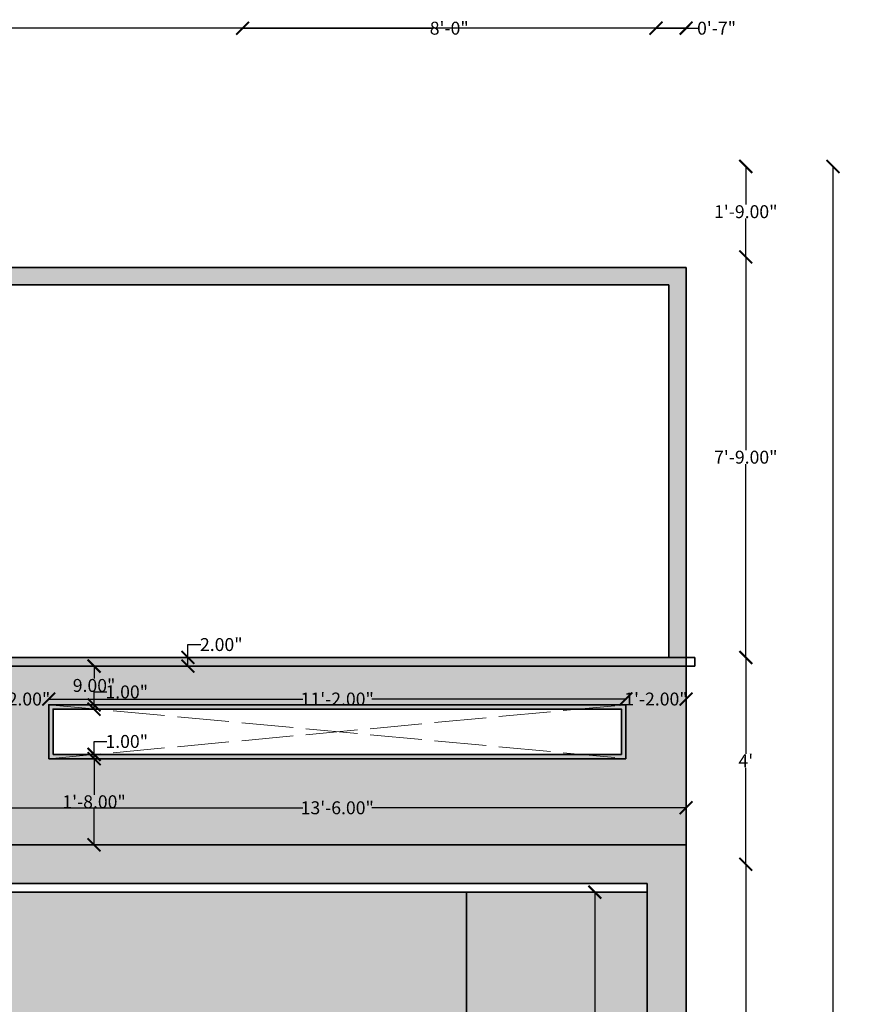
# Model space of a CAD drawing. Units: inches. Extents: x -654 to 390, y -40 to 648.
# Tile 13 of 13: x 192 to 386, y 417 to 645. Entities that reach past the tile are written whole.
import ezdxf

# ---------------------------------------------------------------- set-up
doc = ezdxf.new("R2010")
doc.units = ezdxf.units.IN
doc.header["$PDMODE"] = 3
doc.linetypes.add('ACAD_ISO02W100', pattern=[15, 12, -3])
for name, color, linetype, lineweight in [('A-ANNO-DIMS', 2, 'Continuous', 18), ('A-ELEV', 7, 'Continuous', 35), ('A-ELEV-FILL', 252, 'Continuous', 13), ('A-ELEV-HIDN', 8, 'ACAD_ISO02W100', 18)]:
    doc.layers.add(name, color=color, linetype=linetype, lineweight=lineweight)
doc.styles.get("Standard").update_dxf_attribs({"font": 'arial.ttf'})
doc.dimstyles.get("Standard").update_dxf_attribs({"dimtxt": 3, "dimasz": 3, "dimexe": 0.18, "dimexo": 0.0625, "dimgap": 0.09, "dimtad": 0, "dimtih": 1, "dimtoh": 1, "dimzin": 0, "dimdsep": 46, "dimlunit": 3, "dimtxsty": 'Standard', "dimblk": 'ARCHTICK', "dimcen": 0.09, "dimse1": 1, "dimse2": 1, "dimadec": 0, "dimazin": 0, "dimtfac": 1, "dimtofl": 0, "dimtmove": 0, "dimatfit": 3, "dimfxl": 1, "dimtolj": 1, "dimtzin": 0, "dimarcsym": 0})

# ---------------------------------------------------------------- blocks, each defined once
blk = doc.blocks.new('_ArchTick')
at = {"color": 0, "linetype": 'ByBlock', "const_width": 0.15}
blk.add_lwpolyline([(-0.5, -0.5), (0.5, 0.5)], dxfattribs=at)
blk = doc.blocks.new('*D6')
at = {"layer": 'A-ANNO-DIMS', "color": 0, "lineweight": -2, "transparency": 16777216}
for p, q in [((360.51, 449.13), (360.51, 381.76)), ((360.51, 311.13), (360.51, 378.51))]:
    blk.add_line(p, q, dxfattribs=at)
at = {"layer": 'Defpoints', "color": 0, "transparency": 16777216}
for p in [(337.55, 449.13), (360.51, 449.13), (303.82, 311.13)]:
    blk.add_point(p, dxfattribs=at)
at = {"layer": 'A-ANNO-DIMS', "color": 0, "lineweight": -2, "transparency": 16777216, "xscale": 3, "yscale": 3, "zscale": 3}
for p, rotation in [((360.51, 449.13), 90), ((360.51, 311.13), 270)]:
    blk.add_blockref('_ArchTick', p, dxfattribs=dict(at, rotation=rotation))
at = {"layer": 'A-ANNO-DIMS', "color": 0, "transparency": 16777216, "insert": (360.51, 380.13), "char_height": 3, "attachment_point": 5}
blk.add_mtext('\\A1;11\'-6.00"', dxfattribs=at)
blk = doc.blocks.new('*D7')
at = {"layer": 'A-ANNO-DIMS', "color": 0, "lineweight": -2, "transparency": 16777216}
for p, q in [((360.51, 497.13), (360.51, 474.72)), ((360.51, 449.13), (360.51, 471.54))]:
    blk.add_line(p, q, dxfattribs=at)
at = {"layer": 'Defpoints', "color": 0, "transparency": 16777216}
for p in [(346.65, 497.13), (360.51, 497.13), (337.55, 449.13)]:
    blk.add_point(p, dxfattribs=at)
at = {"layer": 'A-ANNO-DIMS', "color": 0, "lineweight": -2, "transparency": 16777216, "xscale": 3, "yscale": 3, "zscale": 3}
for p, rotation in [((360.51, 497.13), 90), ((360.51, 449.13), 270)]:
    blk.add_blockref('_ArchTick', p, dxfattribs=dict(at, rotation=rotation))
at = {"layer": 'A-ANNO-DIMS', "color": 0, "transparency": 16777216, "insert": (360.51, 473.13), "char_height": 3, "attachment_point": 5}
blk.add_mtext("\\A1;4'", dxfattribs=at)
blk = doc.blocks.new('*D8')
at = {"layer": 'A-ANNO-DIMS', "color": 0, "lineweight": -2, "transparency": 16777216}
for p, q in [((360.51, 590.13), (360.51, 545.26)), ((360.51, 497.13), (360.51, 542.01))]:
    blk.add_line(p, q, dxfattribs=at)
at = {"layer": 'Defpoints', "color": 0, "transparency": 16777216}
for p in [(161.04, 590.13), (360.51, 590.13), (346.65, 497.13)]:
    blk.add_point(p, dxfattribs=at)
at = {"layer": 'A-ANNO-DIMS', "color": 0, "lineweight": -2, "transparency": 16777216, "xscale": 3, "yscale": 3, "zscale": 3}
for p, rotation in [((360.51, 590.13), 90), ((360.51, 497.13), 270)]:
    blk.add_blockref('_ArchTick', p, dxfattribs=dict(at, rotation=rotation))
at = {"layer": 'A-ANNO-DIMS', "color": 0, "transparency": 16777216, "insert": (360.51, 543.63), "char_height": 3, "attachment_point": 5}
blk.add_mtext('\\A1;7\'-9.00"', dxfattribs=at)
blk = doc.blocks.new('*D9')
at = {"layer": 'A-ANNO-DIMS', "color": 0, "lineweight": -2, "transparency": 16777216}
for p, q in [((360.51, 611.13), (360.51, 602.26)), ((360.51, 590.13), (360.51, 599.01))]:
    blk.add_line(p, q, dxfattribs=at)
at = {"layer": 'Defpoints', "color": 0, "transparency": 16777216}
for p in [(126.65, 611.13), (360.51, 611.13), (161.04, 590.13)]:
    blk.add_point(p, dxfattribs=at)
at = {"layer": 'A-ANNO-DIMS', "color": 0, "lineweight": -2, "transparency": 16777216, "xscale": 3, "yscale": 3, "zscale": 3}
for p, rotation in [((360.51, 611.13), 90), ((360.51, 590.13), 270)]:
    blk.add_blockref('_ArchTick', p, dxfattribs=dict(at, rotation=rotation))
at = {"layer": 'A-ANNO-DIMS', "color": 0, "transparency": 16777216, "insert": (360.51, 600.63), "char_height": 3, "attachment_point": 5}
blk.add_mtext('\\A1;1\'-9.00"', dxfattribs=at)
blk = doc.blocks.new('*D32')
at = {"layer": 'A-ANNO-DIMS', "color": 0, "lineweight": -2, "transparency": 16777216}
for p, q in [((184.65, 462.23), (257.63, 462.23)), ((346.65, 462.23), (273.66, 462.23))]:
    blk.add_line(p, q, dxfattribs=at)
at = {"layer": 'Defpoints', "color": 0, "transparency": 16777216}
for p in [(184.65, 462.23), (346.65, 462.23), (346.65, 462.23)]:
    blk.add_point(p, dxfattribs=at)
at = {"layer": 'A-ANNO-DIMS', "color": 0, "lineweight": -2, "transparency": 16777216, "xscale": 3, "yscale": 3, "zscale": 3, "rotation": 180}
blk.add_blockref('_ArchTick', (184.65, 462.23), dxfattribs=at)
at = {"layer": 'A-ANNO-DIMS', "color": 0, "lineweight": -2, "transparency": 16777216, "xscale": 3, "yscale": 3, "zscale": 3}
blk.add_blockref('_ArchTick', (346.65, 462.23), dxfattribs=at)
at = {"layer": 'A-ANNO-DIMS', "color": 0, "transparency": 16777216, "insert": (265.65, 462.23), "char_height": 3, "attachment_point": 5}
blk.add_mtext('\\A1;13\'-6.00"', dxfattribs=at)
blk = doc.blocks.new('*D33')
at = {"layer": 'A-ANNO-DIMS', "color": 0, "lineweight": -2, "transparency": 16777216}
for p, q in [((209.18, 473.63), (209.18, 465.26)), ((209.18, 453.63), (209.18, 462.01))]:
    blk.add_line(p, q, dxfattribs=at)
at = {"layer": 'Defpoints', "color": 0, "transparency": 16777216}
for p in [(198.65, 473.63), (198.65, 453.63), (209.18, 453.63)]:
    blk.add_point(p, dxfattribs=at)
at = {"layer": 'A-ANNO-DIMS', "color": 0, "lineweight": -2, "transparency": 16777216, "xscale": 3, "yscale": 3, "zscale": 3}
for p, rotation in [((209.18, 473.63), 90), ((209.18, 453.63), 270)]:
    blk.add_blockref('_ArchTick', p, dxfattribs=dict(at, rotation=rotation))
at = {"layer": 'A-ANNO-DIMS', "color": 0, "transparency": 16777216, "insert": (209.18, 463.63), "char_height": 3, "attachment_point": 5}
blk.add_mtext('\\A1;1\'-8.00"', dxfattribs=at)
blk = doc.blocks.new('*D34')
at = {"layer": 'A-ANNO-DIMS', "color": 0, "lineweight": -2, "transparency": 16777216}
for p, q in [((209.18, 474.63), (209.18, 477.63)), ((209.18, 477.63), (212.18, 477.63)), ((209.18, 473.63), (209.18, 474.63))]:
    blk.add_line(p, q, dxfattribs=at)
at = {"layer": 'Defpoints', "color": 0, "transparency": 16777216}
for p in [(209.18, 474.63), (209.18, 474.63), (209.18, 473.63)]:
    blk.add_point(p, dxfattribs=at)
at = {"layer": 'A-ANNO-DIMS', "color": 0, "lineweight": -2, "transparency": 16777216, "xscale": 3, "yscale": 3, "zscale": 3}
for p, rotation in [((209.18, 474.63), 90), ((209.18, 473.63), 270)]:
    blk.add_blockref('_ArchTick', p, dxfattribs=dict(at, rotation=rotation))
at = {"layer": 'A-ANNO-DIMS', "color": 0, "transparency": 16777216, "insert": (216.77, 477.63), "char_height": 3, "attachment_point": 5}
blk.add_mtext('\\A1;1.00"', dxfattribs=at)
blk = doc.blocks.new('*D35')
at = {"layer": 'A-ANNO-DIMS', "color": 0, "lineweight": -2, "transparency": 16777216}
for p, q in [((209.18, 486.13), (209.18, 489.13)), ((209.18, 489.13), (212.18, 489.13)), ((209.18, 485.13), (209.18, 486.13))]:
    blk.add_line(p, q, dxfattribs=at)
at = {"layer": 'Defpoints', "color": 0, "transparency": 16777216}
for p in [(209.18, 486.13), (209.37, 486.13), (209.37, 485.13)]:
    blk.add_point(p, dxfattribs=at)
at = {"layer": 'A-ANNO-DIMS', "color": 0, "lineweight": -2, "transparency": 16777216, "xscale": 3, "yscale": 3, "zscale": 3}
for p, rotation in [((209.18, 486.13), 90), ((209.18, 485.13), 270)]:
    blk.add_blockref('_ArchTick', p, dxfattribs=dict(at, rotation=rotation))
at = {"layer": 'A-ANNO-DIMS', "color": 0, "transparency": 16777216, "insert": (216.77, 489.13), "char_height": 3, "attachment_point": 5}
blk.add_mtext('\\A1;1.00"', dxfattribs=at)
blk = doc.blocks.new('*D36')
at = {"layer": 'A-ANNO-DIMS', "color": 0, "lineweight": -2, "transparency": 16777216}
for p, q in [((209.18, 495.13), (209.18, 492.26)), ((209.18, 486.13), (209.18, 489.01))]:
    blk.add_line(p, q, dxfattribs=at)
at = {"layer": 'Defpoints', "color": 0, "transparency": 16777216}
for p in [(198.65, 495.13), (209.18, 495.13), (198.65, 486.13)]:
    blk.add_point(p, dxfattribs=at)
at = {"layer": 'A-ANNO-DIMS', "color": 0, "lineweight": -2, "transparency": 16777216, "xscale": 3, "yscale": 3, "zscale": 3}
for p, rotation in [((209.18, 495.13), 90), ((209.18, 486.13), 270)]:
    blk.add_blockref('_ArchTick', p, dxfattribs=dict(at, rotation=rotation))
at = {"layer": 'A-ANNO-DIMS', "color": 0, "transparency": 16777216, "insert": (209.18, 490.63), "char_height": 3, "attachment_point": 5}
blk.add_mtext('\\A1;9.00"', dxfattribs=at)
blk = doc.blocks.new('*D37')
at = {"layer": 'A-ANNO-DIMS', "color": 0, "lineweight": -2, "transparency": 16777216}
for p, q in [((184.65, 487.48), (184.8, 487.48)), ((198.65, 487.48), (198.5, 487.48))]:
    blk.add_line(p, q, dxfattribs=at)
at = {"layer": 'Defpoints', "color": 0, "transparency": 16777216}
for p in [(184.65, 487.48), (184.65, 486.13), (198.65, 486.13)]:
    blk.add_point(p, dxfattribs=at)
at = {"layer": 'A-ANNO-DIMS', "color": 0, "lineweight": -2, "transparency": 16777216, "xscale": 3, "yscale": 3, "zscale": 3, "rotation": 180}
blk.add_blockref('_ArchTick', (184.65, 487.48), dxfattribs=at)
at = {"layer": 'A-ANNO-DIMS', "color": 0, "lineweight": -2, "transparency": 16777216, "xscale": 3, "yscale": 3, "zscale": 3}
blk.add_blockref('_ArchTick', (198.65, 487.48), dxfattribs=at)
at = {"layer": 'A-ANNO-DIMS', "color": 0, "transparency": 16777216, "insert": (191.65, 487.48), "char_height": 3, "attachment_point": 5}
blk.add_mtext('\\A1;1\'-2.00"', dxfattribs=at)
blk = doc.blocks.new('*D38')
at = {"layer": 'A-ANNO-DIMS', "color": 0, "lineweight": -2, "transparency": 16777216}
for p, q in [((198.65, 487.48), (257.63, 487.48)), ((332.65, 487.48), (273.66, 487.48))]:
    blk.add_line(p, q, dxfattribs=at)
at = {"layer": 'Defpoints', "color": 0, "transparency": 16777216}
for p in [(332.65, 487.48), (198.65, 486.13), (332.65, 486.13)]:
    blk.add_point(p, dxfattribs=at)
at = {"layer": 'A-ANNO-DIMS', "color": 0, "lineweight": -2, "transparency": 16777216, "xscale": 3, "yscale": 3, "zscale": 3, "rotation": 180}
blk.add_blockref('_ArchTick', (198.65, 487.48), dxfattribs=at)
at = {"layer": 'A-ANNO-DIMS', "color": 0, "lineweight": -2, "transparency": 16777216, "xscale": 3, "yscale": 3, "zscale": 3}
blk.add_blockref('_ArchTick', (332.65, 487.48), dxfattribs=at)
at = {"layer": 'A-ANNO-DIMS', "color": 0, "transparency": 16777216, "insert": (265.65, 487.48), "char_height": 3, "attachment_point": 5}
blk.add_mtext('\\A1;11\'-2.00"', dxfattribs=at)
blk = doc.blocks.new('*D39')
at = {"layer": 'A-ANNO-DIMS', "color": 0, "lineweight": -2, "transparency": 16777216}
for p, q in [((332.65, 487.48), (332.8, 487.48)), ((346.65, 487.48), (346.5, 487.48))]:
    blk.add_line(p, q, dxfattribs=at)
at = {"layer": 'Defpoints', "color": 0, "transparency": 16777216}
for p in [(346.65, 487.48), (346.65, 487.48), (332.65, 486.13)]:
    blk.add_point(p, dxfattribs=at)
at = {"layer": 'A-ANNO-DIMS', "color": 0, "lineweight": -2, "transparency": 16777216, "xscale": 3, "yscale": 3, "zscale": 3, "rotation": 180}
blk.add_blockref('_ArchTick', (332.65, 487.48), dxfattribs=at)
at = {"layer": 'A-ANNO-DIMS', "color": 0, "lineweight": -2, "transparency": 16777216, "xscale": 3, "yscale": 3, "zscale": 3}
blk.add_blockref('_ArchTick', (346.65, 487.48), dxfattribs=at)
at = {"layer": 'A-ANNO-DIMS', "color": 0, "transparency": 16777216, "insert": (339.65, 487.48), "char_height": 3, "attachment_point": 5}
blk.add_mtext('\\A1;1\'-2.00"', dxfattribs=at)
blk = doc.blocks.new('*D40')
at = {"layer": 'A-ANNO-DIMS', "color": 0, "lineweight": -2, "transparency": 16777216}
for p, q in [((230.97, 497.13), (230.97, 500.13)), ((230.97, 500.13), (233.97, 500.13)), ((230.97, 495.13), (230.97, 497.13))]:
    blk.add_line(p, q, dxfattribs=at)
at = {"layer": 'Defpoints', "color": 0, "transparency": 16777216}
for p in [(182.52, 497.13), (230.97, 497.13), (182.52, 495.13)]:
    blk.add_point(p, dxfattribs=at)
at = {"layer": 'A-ANNO-DIMS', "color": 0, "lineweight": -2, "transparency": 16777216, "xscale": 3, "yscale": 3, "zscale": 3}
for p, rotation in [((230.97, 497.13), 90), ((230.97, 495.13), 270)]:
    blk.add_blockref('_ArchTick', p, dxfattribs=dict(at, rotation=rotation))
at = {"layer": 'A-ANNO-DIMS', "color": 0, "transparency": 16777216, "insert": (238.72, 500.13), "char_height": 3, "attachment_point": 5}
blk.add_mtext('\\A1;2.00"', dxfattribs=at)
blk = doc.blocks.new('*D41')
at = {"layer": 'A-ANNO-DIMS', "color": 0, "lineweight": -2, "transparency": 16777216}
for p, q in [((325.46, 442.63), (325.46, 311.76)), ((325.46, 177.63), (325.46, 308.51))]:
    blk.add_line(p, q, dxfattribs=at)
at = {"layer": 'Defpoints', "color": 0, "transparency": 16777216}
for p in [(295.65, 442.63), (295.65, 177.63), (325.46, 177.63)]:
    blk.add_point(p, dxfattribs=at)
at = {"layer": 'A-ANNO-DIMS', "color": 0, "lineweight": -2, "transparency": 16777216, "xscale": 3, "yscale": 3, "zscale": 3}
for p, rotation in [((325.46, 442.63), 90), ((325.46, 177.63), 270)]:
    blk.add_blockref('_ArchTick', p, dxfattribs=dict(at, rotation=rotation))
at = {"layer": 'A-ANNO-DIMS', "color": 0, "transparency": 16777216, "insert": (325.46, 310.13), "char_height": 3, "attachment_point": 5}
blk.add_mtext('\\A1;22\'-1.00"', dxfattribs=at)
blk = doc.blocks.new('*D75')
at = {"layer": 'A-ANNO-DIMS', "color": 0, "lineweight": -2, "transparency": 16777216}
for p, q in [((-1.35, 643.23), (167.38, 643.23)), ((346.65, 643.23), (177.91, 643.23))]:
    blk.add_line(p, q, dxfattribs=at)
at = {"layer": 'Defpoints', "color": 0, "transparency": 16777216}
for p in [(346.65, 643.23), (-1.35, 611.13), (346.65, 587.63)]:
    blk.add_point(p, dxfattribs=at)
at = {"layer": 'A-ANNO-DIMS', "color": 0, "lineweight": -2, "transparency": 16777216, "xscale": 3, "yscale": 3, "zscale": 3, "rotation": 180}
blk.add_blockref('_ArchTick', (-1.35, 643.23), dxfattribs=at)
at = {"layer": 'A-ANNO-DIMS', "color": 0, "lineweight": -2, "transparency": 16777216, "xscale": 3, "yscale": 3, "zscale": 3}
blk.add_blockref('_ArchTick', (346.65, 643.23), dxfattribs=at)
at = {"layer": 'A-ANNO-DIMS', "color": 0, "transparency": 16777216, "insert": (172.65, 643.23), "char_height": 3, "attachment_point": 5}
blk.add_mtext('\\A1;29\'-0"', dxfattribs=at)
blk = doc.blocks.new('*D76')
at = {"layer": 'A-ANNO-DIMS', "color": 0, "lineweight": -2, "transparency": 16777216}
for p, q in [((380.75, 611.13), (380.75, 306.76)), ((380.75, -0.87), (380.75, 303.51))]:
    blk.add_line(p, q, dxfattribs=at)
at = {"layer": 'Defpoints', "color": 0, "transparency": 16777216}
for p in [(126.65, 611.13), (380.75, 611.13), (346.65, -0.87)]:
    blk.add_point(p, dxfattribs=at)
at = {"layer": 'A-ANNO-DIMS', "color": 0, "lineweight": -2, "transparency": 16777216, "xscale": 3, "yscale": 3, "zscale": 3}
for p, rotation in [((380.75, 611.13), 90), ((380.75, -0.87), 270)]:
    blk.add_blockref('_ArchTick', p, dxfattribs=dict(at, rotation=rotation))
at = {"layer": 'A-ANNO-DIMS', "color": 0, "transparency": 16777216, "insert": (380.75, 305.13), "char_height": 3, "attachment_point": 5}
blk.add_mtext('\\A1;51\'-0"', dxfattribs=at)
blk = doc.blocks.new('*D89')
at = {"layer": 'A-ANNO-DIMS', "color": 0, "lineweight": -2, "transparency": 16777216}
for p, q in [((243.65, 643.23), (287.57, 643.23)), ((339.65, 643.23), (295.73, 643.23))]:
    blk.add_line(p, q, dxfattribs=at)
at = {"layer": 'Defpoints', "color": 0, "transparency": 16777216}
for p in [(339.65, 643.23), (243.65, 17.13), (339.65, 17.13)]:
    blk.add_point(p, dxfattribs=at)
at = {"layer": 'A-ANNO-DIMS', "color": 0, "lineweight": -2, "transparency": 16777216, "xscale": 3, "yscale": 3, "zscale": 3, "rotation": 180}
blk.add_blockref('_ArchTick', (243.65, 643.23), dxfattribs=at)
at = {"layer": 'A-ANNO-DIMS', "color": 0, "lineweight": -2, "transparency": 16777216, "xscale": 3, "yscale": 3, "zscale": 3}
blk.add_blockref('_ArchTick', (339.65, 643.23), dxfattribs=at)
at = {"layer": 'A-ANNO-DIMS', "color": 0, "transparency": 16777216, "insert": (291.65, 643.23), "char_height": 3, "attachment_point": 5}
blk.add_mtext('\\A1;8\'-0"', dxfattribs=at)
blk = doc.blocks.new('*D90')
at = {"layer": 'A-ANNO-DIMS', "color": 0, "lineweight": -2, "transparency": 16777216}
for p, q in [((339.65, 643.23), (346.65, 643.23)), ((346.65, 643.23), (349.65, 643.23))]:
    blk.add_line(p, q, dxfattribs=at)
at = {"layer": 'Defpoints', "color": 0, "transparency": 16777216}
for p in [(346.65, 643.23), (339.65, 17.13), (346.65, 17.13)]:
    blk.add_point(p, dxfattribs=at)
at = {"layer": 'A-ANNO-DIMS', "color": 0, "lineweight": -2, "transparency": 16777216, "xscale": 3, "yscale": 3, "zscale": 3, "rotation": 180}
blk.add_blockref('_ArchTick', (339.65, 643.23), dxfattribs=at)
at = {"layer": 'A-ANNO-DIMS', "color": 0, "lineweight": -2, "transparency": 16777216, "xscale": 3, "yscale": 3, "zscale": 3}
blk.add_blockref('_ArchTick', (346.65, 643.23), dxfattribs=at)
at = {"layer": 'A-ANNO-DIMS', "color": 0, "transparency": 16777216, "insert": (353.72, 643.23), "char_height": 3, "attachment_point": 5}
blk.add_mtext('\\A1;0\'-7"', dxfattribs=at)

msp = doc.modelspace()

# ---------------------------------------------------------------- hatches: boundary and pattern name
at = {"layer": 'A-ELEV-FILL'}
h = msp.add_hatch(color=256, dxfattribs=at)
h.dxf.hatch_style = 1
h.paths.add_polyline_path([(126.646, 611.134), (124.646, 611.134), (-1.354, 611.134), (-3.354, 611.134), (-3.354, 609.134), (-1.354, 609.134), (124.646, 609.134), (126.646, 609.134)])
h.paths.add_polyline_path([(8.646, 497.134), (-2.354, 497.134), (-2.354, 495.134), (8.646, 495.134)])
h.paths.add_polyline_path([(346.646, 497.134), (182.515, 497.134), (182.515, 495.134), (346.646, 495.134)])
h.paths.add_polyline_path([(198.646, 486.134), (198.646, 473.634), (209.366, 474.634), (199.646, 474.634), (199.646, 485.134), (209.366, 485.134)])
h.paths.add_polyline_path([(332.646, 486.134), (198.646, 486.134), (209.366, 485.134), (321.926, 485.134)])
h.paths.add_polyline_path([(321.926, 474.634), (209.366, 474.634), (198.646, 473.634), (332.646, 473.634)])
h.paths.add_polyline_path([(332.646, 486.134), (321.926, 485.134), (331.646, 485.134), (331.646, 474.634), (321.926, 474.634), (332.646, 473.634)])
h = msp.add_hatch(color=256, dxfattribs=at)
h.dxf.hatch_style = 1
h.paths.add_polyline_path([(161.035, 590.134), (-1.354, 590.134), (-1.354, 581.134), (161.035, 581.134)])
h.paths.add_polyline_path([(346.646, 453.634), (-1.354, 453.634), (-1.354, 444.634), (337.646, 444.634), (337.646, 177.634), (178.742, 177.634), (178.742, 173.134), (176.742, 173.134), (176.742, 177.634), (166.742, 177.634), (166.742, 173.134), (164.742, 173.134), (164.742, 177.634), (154.742, 177.634), (154.742, 173.134), (152.742, 173.134), (152.742, 177.634), (142.742, 177.634), (142.742, 173.134), (140.742, 173.134), (140.742, 177.634), (130.742, 177.634), (130.742, 173.134), (128.742, 173.134), (128.742, 177.634), (115.646, 177.634), (115.646, 168.634), (346.646, 168.634), (346.646, 173.134)])
h.paths.add_polyline_path([(7.646, 87.642), (-1.354, 87.642), (-1.354, 17.134), (7.646, 17.134)])
h.paths.add_polyline_path([(16.396, 116.134), (60.646, 116.134), (60.646, 83.134), (62.646, 83.134), (113.646, 83.134), (115.646, 83.134), (115.646, 125.134), (7.646, 125.134), (7.646, 89.642), (8.146, 89.642), (8.146, 87.642), (7.646, 87.642), (7.646, 83.134), (9.646, 83.134), (16.396, 83.134)])
h = msp.add_hatch(color=256, dxfattribs=at)
h.dxf.hatch_style = 1
h.paths.add_polyline_path([(346.646, 587.634), (161.035, 587.634), (161.035, 583.634), (342.646, 583.634), (342.646, 497.134), (346.646, 497.134), (346.646, 583.634)])
h.paths.add_polyline_path([(295.646, 315.634), (98.293, 315.634), (98.293, 311.134), (295.646, 311.134)])
h.paths.add_polyline_path([(128.742, 311.134), (98.293, 311.134), (98.293, 306.634), (128.742, 306.634)])
h.paths.add_polyline_path([(140.742, 311.134), (130.742, 311.134), (130.742, 306.634), (140.742, 306.634)])
h.paths.add_polyline_path([(152.742, 311.134), (142.742, 311.134), (142.742, 306.634), (152.742, 306.634)])
h.paths.add_polyline_path([(164.742, 311.134), (154.742, 311.134), (154.742, 306.634), (164.742, 306.634)])
h.paths.add_polyline_path([(176.742, 311.134), (166.742, 311.134), (166.742, 306.634), (176.742, 306.634)])
h.paths.add_polyline_path([(295.646, 311.134), (178.742, 311.134), (178.742, 306.634), (295.646, 306.634)])
h.paths.add_polyline_path([(303.818, 315.634), (295.646, 315.634), (295.646, 311.134), (303.818, 311.134)])
h.paths.add_polyline_path([(303.818, 311.134), (295.646, 311.134), (295.646, 306.634), (303.818, 306.634)])
h = msp.add_hatch(color=256, dxfattribs=at)
h.dxf.hatch_style = 1
h.paths.add_polyline_path([(41.55, 80.08), (28.05, 80.08), (28.05, 20.08), (41.55, 20.08)])
h.paths.add_polyline_path([(93.843, 80.08), (80.343, 80.08), (80.343, 20.08), (93.843, 20.08)])
h.paths.add_polyline_path([(337.646, 442.634), (295.646, 442.634), (295.646, 316.634), (304.646, 316.634), (304.646, 315.634), (303.818, 315.634), (303.818, 306.634), (304.646, 306.634), (304.646, 305.634), (295.646, 305.634), (295.646, 177.634), (337.646, 177.634)])
h.paths.add_polyline_path([(346.646, 495.134), (184.646, 495.134), (184.646, 453.634), (346.646, 453.634)])
h.paths.add_polyline_path([(198.646, 473.634), (198.646, 486.134), (332.646, 486.134), (332.646, 473.634)], flags=16)
h.paths.add_polyline_path([(199.646, 474.634), (199.646, 485.134), (331.646, 485.134), (331.646, 474.634)], flags=0)
h = msp.add_hatch(color=256, dxfattribs=at)
h.dxf.hatch_style = 1
h.paths.add_polyline_path([(239.871, 410.786), (291.141, 410.786), (291.141, 355.634), (295.646, 355.634), (295.646, 442.634), (145.646, 442.634), (145.646, 410.786), (179.877, 410.786), (179.877, 355.634), (239.871, 355.634)])

# ---------------------------------------------------------------- linework, layer by layer
at = {"layer": 'A-ELEV'}
for p, q in [((161.035, 587.634), (346.646, 587.634)), ((346.646, -0.866), (346.646, 587.634)), ((161.035, 583.634), (342.646, 583.634)), ((342.646, 583.634), (342.646, 497.134)), ((346.646, 583.634), (346.646, 497.134)), ((182.515, 497.134), (348.646, 497.134)), ((348.646, 495.134), (348.646, 497.134)), ((182.515, 495.134), (348.646, 495.134)), ((-1.354, 453.634), (346.646, 453.634)), ((-1.354, 444.634), (337.646, 444.634)), ((337.646, 444.634), (337.646, 177.634)), ((-1.354, 442.634), (337.646, 442.634)), ((295.646, 442.634), (295.646, 177.634))]:
    msp.add_line(p, q, dxfattribs=at)
for points in [[(198.646, 473.634), (198.646, 486.134), (332.646, 486.134), (332.646, 473.634)], [(199.646, 474.634), (199.646, 485.134), (331.646, 485.134), (331.646, 474.634)]]:
    msp.add_lwpolyline(points, close=True, dxfattribs=at)
at = {"layer": 'A-ELEV-HIDN'}
for p, q in [((198.646, 486.134), (332.646, 473.634)), ((198.646, 473.634), (332.646, 486.134))]:
    msp.add_line(p, q, dxfattribs=at)

# ---------------------------------------------------------------- dimensions: what is measured, and where the dimension line sits
at = {"layer": 'A-ANNO-DIMS'}
for base, p1, p2, override, picture, middle in [((346.646, 643.234), (-1.354, 611.134), (346.646, 587.634), {"dimdec": 1, "dimlfac": 1, "dimrnd": 0, "dimzin": 1, "dimdsep": 46, "dimlunit": 4, "dimfrac": 2}, '*D75', (172.646, 643.234)), ((339.646, 643.234), (243.646, 17.134), (339.646, 17.134), {"dimdec": 1, "dimlfac": 1, "dimrnd": 0, "dimzin": 1, "dimdsep": 46, "dimlunit": 4, "dimfrac": 2}, '*D89', (291.646, 643.234)), ((346.646, 643.234), (339.646, 17.134), (346.646, 17.134), {"dimdec": 1, "dimlfac": 1, "dimrnd": 0, "dimzin": 1, "dimdsep": 46, "dimlunit": 4, "dimfrac": 2}, '*D90', (353.724, 643.234)), ((184.646, 487.476), (198.646, 486.134), (184.646, 486.134), {"dimclrd": 0, "dimclre": 0, "dimclrt": 0}, '*D37', (191.646, 487.476)), ((332.646, 487.476), (198.646, 486.134), (332.646, 486.134), {"dimclrd": 0, "dimclre": 0, "dimclrt": 0}, '*D38', (265.646, 487.476)), ((346.646, 487.476), (332.646, 486.134), (346.646, 487.476), {"dimclrd": 0, "dimclre": 0, "dimclrt": 0, "dimtmove": 1}, '*D39', (339.646, 487.476)), ((346.646, 462.232), (184.646, 462.232), (346.646, 462.232), {"dimclrd": 0, "dimclre": 0, "dimclrt": 0, "dimtmove": 1}, '*D32', (265.646, 462.232))]:
    dim = msp.add_linear_dim(base=base, p1=p1, p2=p2, dimstyle='Standard', override=override, dxfattribs=at)
    dim.commit()
    dim.dimension.update_dxf_attribs({"geometry": picture, "text_midpoint": middle})
for base, p1, p2, override, picture, middle in [((360.508, 611.134), (161.035, 590.134), (126.646, 611.134), {"dimclrd": 0, "dimclre": 0, "dimclrt": 0, "dimtmove": 1}, '*D9', (360.508, 600.634)), ((380.746, 611.134), (346.646, -0.866), (126.646, 611.134), {"dimdec": 1, "dimlfac": 1, "dimrnd": 0, "dimzin": 1, "dimdsep": 46, "dimlunit": 4, "dimfrac": 2}, '*D76', (380.746, 305.134)), ((360.508, 590.134), (346.646, 497.134), (161.035, 590.134), {"dimclrd": 0, "dimclre": 0, "dimclrt": 0, "dimtmove": 1}, '*D8', (360.508, 543.634)), ((230.972, 497.134), (182.515, 495.134), (182.515, 497.134), {"dimclrd": 0, "dimclre": 0, "dimclrt": 0}, '*D40', (238.724, 500.134)), ((360.508, 497.134), (337.554, 449.134), (346.646, 497.134), {"dimclrd": 0, "dimclre": 0, "dimclrt": 0, "dimtmove": 1}, '*D7', (360.508, 473.134)), ((209.184, 495.134), (198.646, 486.134), (198.646, 495.134), {"dimclrd": 0, "dimclre": 0, "dimclrt": 0}, '*D36', (209.184, 490.634)), ((209.184, 486.134), (209.366, 485.134), (209.366, 486.134), {"dimclrd": 0, "dimclre": 0, "dimclrt": 0}, '*D35', (216.77, 489.134)), ((209.184, 474.634), (209.184, 473.634), (209.184, 474.634), {"dimclrd": 0, "dimclre": 0, "dimclrt": 0}, '*D34', (216.77, 477.634)), ((209.184, 453.634), (198.646, 473.634), (198.646, 453.634), {"dimclrd": 0, "dimclre": 0, "dimclrt": 0}, '*D33', (209.184, 463.634)), ((360.508, 449.134), (303.818, 311.134), (337.554, 449.134), {"dimclrd": 0, "dimclre": 0, "dimclrt": 0, "dimtmove": 1}, '*D6', (360.508, 380.134)), ((325.461, 177.634), (295.646, 442.634), (295.646, 177.634), {"dimclrd": 0, "dimclre": 0, "dimclrt": 0}, '*D41', (325.461, 310.134))]:
    dim = msp.add_linear_dim(base=base, p1=p1, p2=p2, angle=90, dimstyle='Standard', override=override, dxfattribs=at)
    dim.commit()
    dim.dimension.update_dxf_attribs({"geometry": picture, "text_midpoint": middle})

doc.saveas('drawing.dxf')
